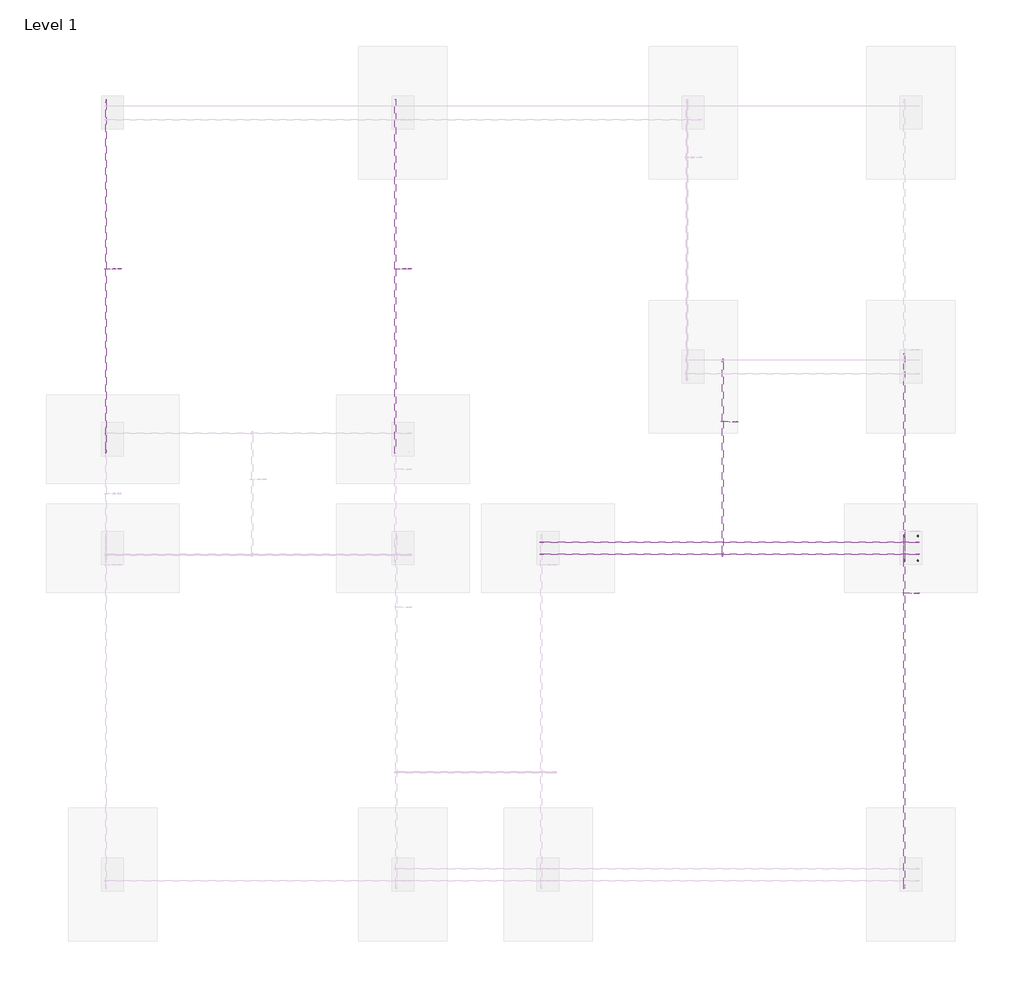
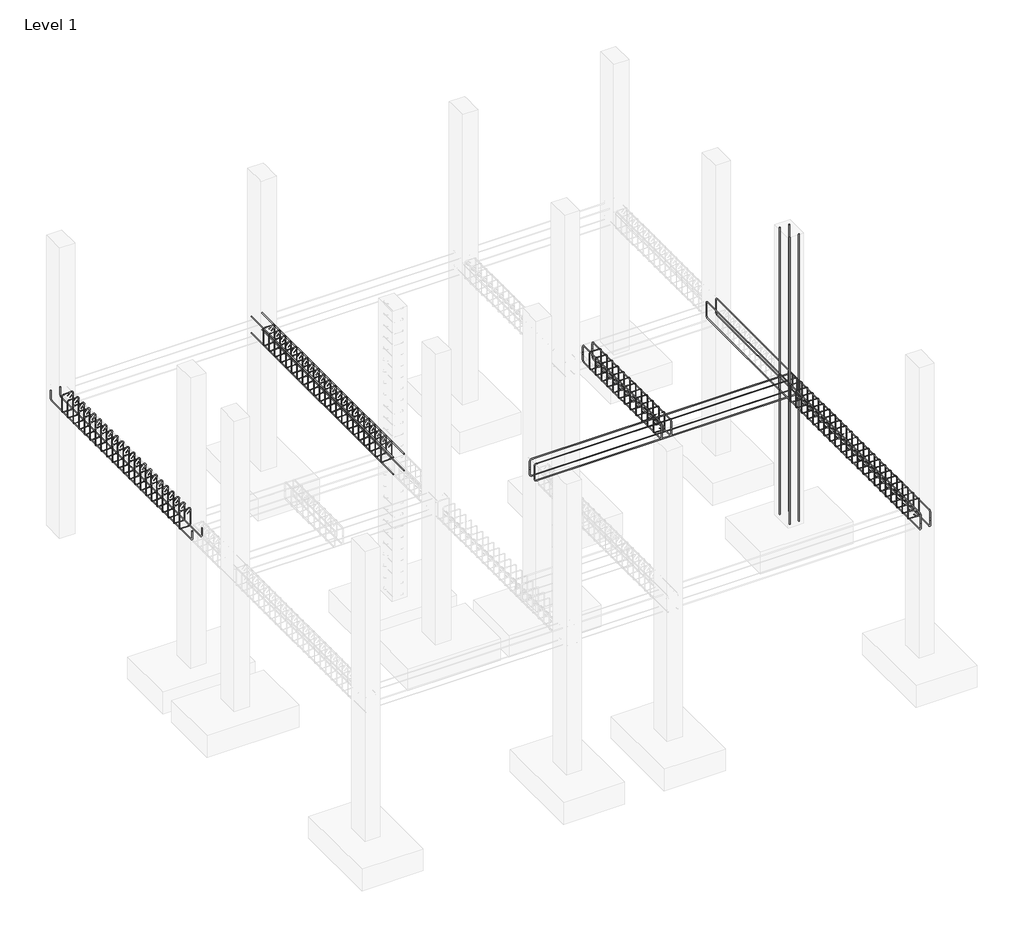
# One storey, part 4 of 5: 17 reinforcing bars.
"""IFC4 building model written with IfcOpenShell, lengths in millimetres."""

from ifc_helpers import new_model, si_unit, point, frame, origin, place, context, project, spatial, polyline, circle_curve, trimmed, segment, composite_curve, source, transform, mapped, element, save
from ifc_brep_helpers import swept_disk

model = new_model("IFC4")

# Units and contexts
model_context = context("Model", 3, world=origin())
ifc_project = project(units=[si_unit("LENGTHUNIT", "METRE", prefix="MILLI")], contexts=[model_context])

# Site, building, storey
site = spatial("IfcSite", under=ifc_project)
building = spatial("IfcBuilding", under=site)
storey = spatial("IfcBuildingStorey", under=building, Name="Level 1", Elevation=0.0)

# Reinforcing bars
placement = place(None, origin())
reinforcing_bar_shape = source(origin(), model_context, "Body", "SolidModel", [
    swept_disk(composite_curve([segment(polyline([(-4212.455746, 5062.3577522, 2793.8967919), (-4212.455746, 5062.3577522, 2946.2967919)]), True, "CONTINUOUS"), segment(trimmed(circle_curve(frame((-4212.455746, 5018.2887522, 2946.2967919), z_axis=(1.0, 0.0, 0.0), x_axis=(0.0, 44.068999999999505, 0.0)), 44.069), [point((-4212.455746, 5062.3577522, 2946.2967919))], [point((-4212.455746, 5018.2887522, 2990.3657919))], True, "CARTESIAN"), True, "CONTINUOUS"), segment(polyline([(-4212.455746, 5018.2887522, 2990.3657919), (-4212.455746, 2237.3647522, 2990.3657919)]), True, "CONTINUOUS"), segment(trimmed(circle_curve(frame((-4212.455746, 2237.3647522, 2946.2967919), z_axis=(1.0, 0.0, 0.0), x_axis=(0.0, 0.0, 44.069000000000415)), 44.069), [point((-4212.455746, 2237.3647522, 2990.3657919))], [point((-4212.455746, 2193.2957522, 2946.2967919))], True, "CARTESIAN"), True, "CONTINUOUS"), segment(polyline([(-4212.455746, 2193.2957522, 2946.2967919), (-4212.455746, 2193.2957522, 2793.8967919)]), True, "CONTINUOUS")], self_intersect=False), 5.969),
])
element("IfcReinforcingBar", 1, at=placement, inside=storey, context=model_context, shape_type="MappedRepresentation", body=[
    mapped(reinforcing_bar_shape, transform((0.0, 0.0, 0.0), x_axis=(1.0, 0.0, 0.0), y_axis=(0.0, 1.0, 0.0), z_axis=(0.0, 0.0, 1.0))),
    mapped(reinforcing_bar_shape, transform((-189.5315837, 0.0, 0.0), x_axis=(1.0, 0.0, 0.0), y_axis=(0.0, 1.0, 0.0), z_axis=(0.0, 0.0, 1.0))),
])
reinforcing_bar_2_shape = source(origin(), model_context, "Body", "SolidModel", [
    swept_disk(composite_curve([segment(polyline([(-4212.455746, 2193.2957522, 2844.9032081), (-4212.455746, 2193.2957522, 2692.5032081)]), True, "CONTINUOUS"), segment(trimmed(circle_curve(frame((-4212.455746, 2237.3647522, 2692.5032081), z_axis=(1.0, 0.0, 0.0), x_axis=(0.0, -44.06899999999996, 0.0)), 44.069), [point((-4212.455746, 2193.2957522, 2692.5032081))], [point((-4212.455746, 2237.3647522, 2648.4342081))], True, "CARTESIAN"), True, "CONTINUOUS"), segment(polyline([(-4212.455746, 2237.3647522, 2648.4342081), (-4212.455746, 5018.2887522, 2648.4342081)]), True, "CONTINUOUS"), segment(trimmed(circle_curve(frame((-4212.455746, 5018.2887522, 2692.5032081), z_axis=(1.0, 0.0, 0.0), x_axis=(0.0, 0.0, -44.06899999999996)), 44.069), [point((-4212.455746, 5018.2887522, 2648.4342081))], [point((-4212.455746, 5062.3577522, 2692.5032081))], True, "CARTESIAN"), True, "CONTINUOUS"), segment(polyline([(-4212.455746, 5062.3577522, 2692.5032081), (-4212.455746, 5062.3577522, 2844.9032081)]), True, "CONTINUOUS")], self_intersect=False), 5.969),
])
element("IfcReinforcingBar", 2, at=placement, inside=storey, context=model_context, shape_type="MappedRepresentation", body=[
    mapped(reinforcing_bar_2_shape, transform((0.0, 0.0, 0.0), x_axis=(1.0, 0.0, 0.0), y_axis=(0.0, 1.0, 0.0), z_axis=(0.0, 0.0, 1.0))),
    mapped(reinforcing_bar_2_shape, transform((-189.5315837, 0.0, 0.0), x_axis=(1.0, 0.0, 0.0), y_axis=(0.0, 1.0, 0.0), z_axis=(0.0, 0.0, 1.0))),
])
reinforcing_bar_3_shape = source(origin(), model_context, "Body", "SolidModel", [
    swept_disk(composite_curve([segment(polyline([(-4212.455746, 2562.3577522, 2793.8967919), (-4212.455746, 2562.3577522, 2946.2967919)]), True, "CONTINUOUS"), segment(trimmed(circle_curve(frame((-4212.455746, 2518.2887522, 2946.2967919), z_axis=(1.0, 0.0, 0.0), x_axis=(0.0, 44.06899999999996, 0.0)), 44.069), [point((-4212.455746, 2562.3577522, 2946.2967919))], [point((-4212.455746, 2518.2887522, 2990.3657919))], True, "CARTESIAN"), True, "CONTINUOUS"), segment(polyline([(-4212.455746, 2518.2887522, 2990.3657919), (-4212.455746, -2262.6352478, 2990.3657919)]), True, "CONTINUOUS"), segment(trimmed(circle_curve(frame((-4212.455746, -2262.6352478, 2946.2967919), z_axis=(1.0, 0.0, 0.0), x_axis=(0.0, 0.0, 44.069000000000415)), 44.069), [point((-4212.455746, -2262.6352478, 2990.3657919))], [point((-4212.455746, -2306.7042478, 2946.2967919))], True, "CARTESIAN"), True, "CONTINUOUS"), segment(polyline([(-4212.455746, -2306.7042478, 2946.2967919), (-4212.455746, -2306.7042478, 2793.8967919)]), True, "CONTINUOUS")], self_intersect=False), 5.969),
])
element("IfcReinforcingBar", 3, at=placement, inside=storey, context=model_context, shape_type="MappedRepresentation", body=[
    mapped(reinforcing_bar_3_shape, transform((0.0, 0.0, 0.0), x_axis=(1.0, 0.0, 0.0), y_axis=(0.0, 1.0, 0.0), z_axis=(0.0, 0.0, 1.0))),
    mapped(reinforcing_bar_3_shape, transform((-189.5315837, 0.0, 0.0), x_axis=(1.0, 0.0, 0.0), y_axis=(0.0, 1.0, 0.0), z_axis=(0.0, 0.0, 1.0))),
])
reinforcing_bar_4_shape = source(origin(), model_context, "Body", "SolidModel", [
    swept_disk(composite_curve([segment(polyline([(-4212.455746, -2306.7042478, 2844.9032081), (-4212.455746, -2306.7042478, 2692.5032081)]), True, "CONTINUOUS"), segment(trimmed(circle_curve(frame((-4212.455746, -2262.6352478, 2692.5032081), z_axis=(1.0, 0.0, 0.0), x_axis=(0.0, -44.06899999999996, 0.0)), 44.069), [point((-4212.455746, -2306.7042478, 2692.5032081))], [point((-4212.455746, -2262.6352478, 2648.4342081))], True, "CARTESIAN"), True, "CONTINUOUS"), segment(polyline([(-4212.455746, -2262.6352478, 2648.4342081), (-4212.455746, 2518.2887522, 2648.4342081)]), True, "CONTINUOUS"), segment(trimmed(circle_curve(frame((-4212.455746, 2518.2887522, 2692.5032081), z_axis=(1.0, 0.0, 0.0), x_axis=(0.0, 0.0, -44.06899999999996)), 44.069), [point((-4212.455746, 2518.2887522, 2648.4342081))], [point((-4212.455746, 2562.3577522, 2692.5032081))], True, "CARTESIAN"), True, "CONTINUOUS"), segment(polyline([(-4212.455746, 2562.3577522, 2692.5032081), (-4212.455746, 2562.3577522, 2844.9032081)]), True, "CONTINUOUS")], self_intersect=False), 5.969),
])
element("IfcReinforcingBar", 4, at=placement, inside=storey, context=model_context, shape_type="MappedRepresentation", body=[
    mapped(reinforcing_bar_4_shape, transform((0.0, 0.0, 0.0), x_axis=(1.0, 0.0, 0.0), y_axis=(0.0, 1.0, 0.0), z_axis=(0.0, 0.0, 1.0))),
    mapped(reinforcing_bar_4_shape, transform((-189.5315837, 0.0, 0.0), x_axis=(1.0, 0.0, 0.0), y_axis=(0.0, 1.0, 0.0), z_axis=(0.0, 0.0, 1.0))),
])
reinforcing_bar_5_shape = source(origin(), model_context, "Body", "SolidModel", [
    swept_disk(composite_curve([segment(polyline([(-4213.892587, 2547.3557031, 38.1), (-4213.892587, 2547.3557031, 6057.9)]), True, "CONTINUOUS")], self_intersect=False), 8.001),
])
element("IfcReinforcingBar", 5, at=placement, inside=storey, context=model_context, shape_type="MappedRepresentation", body=[
    mapped(reinforcing_bar_5_shape, transform((0.0, 0.0, 0.0), x_axis=(1.0, 0.0, 0.0), y_axis=(0.0, 1.0, 0.0), z_axis=(0.0, 0.0, 1.0))),
    mapped(reinforcing_bar_5_shape, transform((-186.6579018, 0.0, 0.0), x_axis=(1.0, 0.0, 0.0), y_axis=(0.0, 1.0, 0.0), z_axis=(0.0, 0.0, 1.0))),
])
reinforcing_bar_6_shape = source(origin(), model_context, "Body", "SolidModel", [
    swept_disk(composite_curve([segment(polyline([(-4213.892587, 2208.2978013, 6057.9), (-4213.892587, 2208.2978013, 38.1)]), True, "CONTINUOUS")], self_intersect=False), 8.001),
])
element("IfcReinforcingBar", 6, at=placement, inside=storey, context=model_context, shape_type="MappedRepresentation", body=[
    mapped(reinforcing_bar_6_shape, transform((0.0, 0.0, 0.0), x_axis=(1.0, 0.0, 0.0), y_axis=(0.0, 1.0, 0.0), z_axis=(0.0, 0.0, 1.0))),
    mapped(reinforcing_bar_6_shape, transform((-186.6579018, 0.0, 0.0), x_axis=(1.0, 0.0, 0.0), y_axis=(0.0, 1.0, 0.0), z_axis=(0.0, 0.0, 1.0))),
])
reinforcing_bar_7_shape = source(origin(), model_context, "Body", "SolidModel", [
    swept_disk(composite_curve([segment(polyline([(-4260.3161447, -1889.6362478, 2737.7833901), (-4205.4511463, -1889.6362478, 2682.9183916)]), True, "CONTINUOUS"), segment(trimmed(circle_curve(frame((-4226.1955379, -1889.6362478, 2662.174), z_axis=(0.0, 1.0, 0.0), x_axis=(20.7443916000002, 0.0, 20.7443916000002)), 29.337), [point((-4205.4511463, -1889.6362478, 2682.9183916))], [point((-4226.1955379, -1889.6362478, 2632.837))], True, "CARTESIAN"), True, "CONTINUOUS"), segment(polyline([(-4226.1955379, -1889.6362478, 2632.837), (-4388.2475379, -1889.6362478, 2632.837)]), True, "CONTINUOUS"), segment(trimmed(circle_curve(frame((-4388.2475379, -1889.6362478, 2662.174), z_axis=(0.0, 1.0, 0.0), x_axis=(0.0, 0.0, -29.33699999999999)), 29.337), [point((-4388.2475379, -1889.6362478, 2632.837))], [point((-4417.5845379, -1889.6362478, 2662.174))], True, "CARTESIAN"), True, "CONTINUOUS"), segment(polyline([(-4417.5845379, -1889.6362478, 2662.174), (-4417.5845379, -1889.6362478, 2976.626)]), True, "CONTINUOUS"), segment(trimmed(circle_curve(frame((-4388.2661869, -1890.6821269, 2976.626), z_axis=(0.03565051078635361, 0.9993643184948481, 0.0), x_axis=(-29.318350999999893, 1.0458790999998655, 0.0)), 29.337), [point((-4417.5845379, -1889.6362478, 2976.626))], [point((-4388.2661869, -1890.6821269, 3005.963))], True, "CARTESIAN"), True, "CONTINUOUS"), segment(polyline([(-4388.2661869, -1890.6821269, 3005.963), (-4226.1768889, -1896.4643688, 3005.963)]), True, "CONTINUOUS"), segment(trimmed(circle_curve(frame((-4226.1768889, -1896.4643688, 2976.626), z_axis=(0.03565051078635361, 0.9993643184948481, 0.0), x_axis=(0.0, 0.0, 29.33699999999999)), 29.337), [point((-4226.1768889, -1896.4643688, 3005.963))], [point((-4196.8585379, -1897.5102478, 2976.626))], True, "CARTESIAN"), True, "CONTINUOUS"), segment(polyline([(-4196.8585379, -1897.5102478, 2976.626), (-4196.8585379, -1897.5102478, 2662.174)]), True, "CONTINUOUS"), segment(trimmed(circle_curve(frame((-4226.1955379, -1897.5102478, 2662.174), z_axis=(0.0, 1.0, 0.0), x_axis=(29.337000000000444, 0.0, 0.0)), 29.337), [point((-4196.8585379, -1897.5102478, 2662.174))], [point((-4246.9399295, -1897.5102478, 2641.4296084))], True, "CARTESIAN"), True, "CONTINUOUS"), segment(polyline([(-4246.9399295, -1897.5102478, 2641.4296084), (-4301.804928, -1897.5102478, 2696.2946068)]), True, "CONTINUOUS")], self_intersect=False), 3.937),
])
element("IfcReinforcingBar", 7, at=placement, inside=storey, context=model_context, shape_type="MappedRepresentation", body=[
    mapped(reinforcing_bar_7_shape, transform((0.0, 0.0, 0.0), x_axis=(1.0, 0.0, 0.0), y_axis=(0.0, 1.0, 0.0), z_axis=(0.0, 0.0, 1.0))),
    mapped(reinforcing_bar_7_shape, transform((0.0, 192.1393333, 0.0), x_axis=(1.0, 0.0, 0.0), y_axis=(0.0, 1.0, 0.0), z_axis=(0.0, 0.0, 1.0))),
    mapped(reinforcing_bar_7_shape, transform((0.0, 384.2786667, 0.0), x_axis=(1.0, 0.0, 0.0), y_axis=(0.0, 1.0, 0.0), z_axis=(0.0, 0.0, 1.0))),
    mapped(reinforcing_bar_7_shape, transform((0.0, 576.418, 0.0), x_axis=(1.0, 0.0, 0.0), y_axis=(0.0, 1.0, 0.0), z_axis=(0.0, 0.0, 1.0))),
    mapped(reinforcing_bar_7_shape, transform((0.0, 768.5573333, 0.0), x_axis=(1.0, 0.0, 0.0), y_axis=(0.0, 1.0, 0.0), z_axis=(0.0, 0.0, 1.0))),
    mapped(reinforcing_bar_7_shape, transform((0.0, 960.6966667, 0.0), x_axis=(1.0, 0.0, 0.0), y_axis=(0.0, 1.0, 0.0), z_axis=(0.0, 0.0, 1.0))),
    mapped(reinforcing_bar_7_shape, transform((0.0, 1152.836, 0.0), x_axis=(1.0, 0.0, 0.0), y_axis=(0.0, 1.0, 0.0), z_axis=(0.0, 0.0, 1.0))),
    mapped(reinforcing_bar_7_shape, transform((0.0, 1344.9753333, 0.0), x_axis=(1.0, 0.0, 0.0), y_axis=(0.0, 1.0, 0.0), z_axis=(0.0, 0.0, 1.0))),
    mapped(reinforcing_bar_7_shape, transform((0.0, 1537.1146667, 0.0), x_axis=(1.0, 0.0, 0.0), y_axis=(0.0, 1.0, 0.0), z_axis=(0.0, 0.0, 1.0))),
    mapped(reinforcing_bar_7_shape, transform((0.0, 1729.254, 0.0), x_axis=(1.0, 0.0, 0.0), y_axis=(0.0, 1.0, 0.0), z_axis=(0.0, 0.0, 1.0))),
    mapped(reinforcing_bar_7_shape, transform((0.0, 1921.3933333, 0.0), x_axis=(1.0, 0.0, 0.0), y_axis=(0.0, 1.0, 0.0), z_axis=(0.0, 0.0, 1.0))),
    mapped(reinforcing_bar_7_shape, transform((0.0, 2113.5326667, 0.0), x_axis=(1.0, 0.0, 0.0), y_axis=(0.0, 1.0, 0.0), z_axis=(0.0, 0.0, 1.0))),
    mapped(reinforcing_bar_7_shape, transform((0.0, 2305.672, 0.0), x_axis=(1.0, 0.0, 0.0), y_axis=(0.0, 1.0, 0.0), z_axis=(0.0, 0.0, 1.0))),
    mapped(reinforcing_bar_7_shape, transform((0.0, 2497.8113333, 0.0), x_axis=(1.0, 0.0, 0.0), y_axis=(0.0, 1.0, 0.0), z_axis=(0.0, 0.0, 1.0))),
    mapped(reinforcing_bar_7_shape, transform((0.0, 2689.9506667, 0.0), x_axis=(1.0, 0.0, 0.0), y_axis=(0.0, 1.0, 0.0), z_axis=(0.0, 0.0, 1.0))),
    mapped(reinforcing_bar_7_shape, transform((0.0, 2882.09, 0.0), x_axis=(1.0, 0.0, 0.0), y_axis=(0.0, 1.0, 0.0), z_axis=(0.0, 0.0, 1.0))),
    mapped(reinforcing_bar_7_shape, transform((0.0, 3074.2293333, 0.0), x_axis=(1.0, 0.0, 0.0), y_axis=(0.0, 1.0, 0.0), z_axis=(0.0, 0.0, 1.0))),
    mapped(reinforcing_bar_7_shape, transform((0.0, 3266.3686667, 0.0), x_axis=(1.0, 0.0, 0.0), y_axis=(0.0, 1.0, 0.0), z_axis=(0.0, 0.0, 1.0))),
    mapped(reinforcing_bar_7_shape, transform((0.0, 3458.508, 0.0), x_axis=(1.0, 0.0, 0.0), y_axis=(0.0, 1.0, 0.0), z_axis=(0.0, 0.0, 1.0))),
    mapped(reinforcing_bar_7_shape, transform((0.0, 3650.6473333, 0.0), x_axis=(1.0, 0.0, 0.0), y_axis=(0.0, 1.0, 0.0), z_axis=(0.0, 0.0, 1.0))),
    mapped(reinforcing_bar_7_shape, transform((0.0, 3842.7866667, 0.0), x_axis=(1.0, 0.0, 0.0), y_axis=(0.0, 1.0, 0.0), z_axis=(0.0, 0.0, 1.0))),
    mapped(reinforcing_bar_7_shape, transform((0.0, 4034.926, 0.0), x_axis=(1.0, 0.0, 0.0), y_axis=(0.0, 1.0, 0.0), z_axis=(0.0, 0.0, 1.0))),
])
reinforcing_bar_8_shape = source(origin(), model_context, "Body", "SolidModel", [
    swept_disk(composite_curve([segment(polyline([(-15212.455746, 3693.2957522, 2844.9032081), (-15212.455746, 3693.2957522, 2692.5032081)]), True, "CONTINUOUS"), segment(trimmed(circle_curve(frame((-15212.455746, 3737.3647522, 2692.5032081), z_axis=(1.0, 0.0, 0.0), x_axis=(0.0, -44.06899999999996, 0.0)), 44.069), [point((-15212.455746, 3693.2957522, 2692.5032081))], [point((-15212.455746, 3737.3647522, 2648.4342081))], True, "CARTESIAN"), True, "CONTINUOUS"), segment(polyline([(-15212.455746, 3737.3647522, 2648.4342081), (-15212.455746, 8518.2887522, 2648.4342081)]), True, "CONTINUOUS"), segment(trimmed(circle_curve(frame((-15212.455746, 8518.2887522, 2692.5032081), z_axis=(1.0, 0.0, 0.0), x_axis=(0.0, 0.0, -44.06899999999996)), 44.069), [point((-15212.455746, 8518.2887522, 2648.4342081))], [point((-15212.455746, 8562.3577522, 2692.5032081))], True, "CARTESIAN"), True, "CONTINUOUS"), segment(polyline([(-15212.455746, 8562.3577522, 2692.5032081), (-15212.455746, 8562.3577522, 2844.9032081)]), True, "CONTINUOUS")], self_intersect=False), 5.969),
])
element("IfcReinforcingBar", 8, at=placement, inside=storey, context=model_context, shape_type="MappedRepresentation", body=[
    mapped(reinforcing_bar_8_shape, transform((0.0, 0.0, 0.0), x_axis=(1.0, 0.0, 0.0), y_axis=(0.0, 1.0, 0.0), z_axis=(0.0, 0.0, 1.0))),
    mapped(reinforcing_bar_8_shape, transform((-189.5315837, 0.0, 0.0), x_axis=(1.0, 0.0, 0.0), y_axis=(0.0, 1.0, 0.0), z_axis=(0.0, 0.0, 1.0))),
])
reinforcing_bar_9_shape = source(origin(), model_context, "Body", "SolidModel", [
    swept_disk(composite_curve([segment(polyline([(-15260.3161447, 8145.2897522, 2901.0166099), (-15205.4511463, 8145.2897522, 2955.8816084)]), True, "CONTINUOUS"), segment(trimmed(circle_curve(frame((-15226.1955379, 8145.2897522, 2976.626), z_axis=(0.0, -1.0, 0.0), x_axis=(20.74439159999929, 0.0, -20.7443916000002)), 29.337), [point((-15205.4511463, 8145.2897522, 2955.8816084))], [point((-15226.1955379, 8145.2897522, 3005.963))], True, "CARTESIAN"), True, "CONTINUOUS"), segment(polyline([(-15226.1955379, 8145.2897522, 3005.963), (-15388.2475379, 8145.2897522, 3005.963)]), True, "CONTINUOUS"), segment(trimmed(circle_curve(frame((-15388.2475379, 8145.2897522, 2976.626), z_axis=(0.0, -1.0, 0.0), x_axis=(0.0, 0.0, 29.33699999999999)), 29.337), [point((-15388.2475379, 8145.2897522, 3005.963))], [point((-15417.5845379, 8145.2897522, 2976.626))], True, "CARTESIAN"), True, "CONTINUOUS"), segment(polyline([(-15417.5845379, 8145.2897522, 2976.626), (-15417.5845379, 8145.2897522, 2662.174)]), True, "CONTINUOUS"), segment(trimmed(circle_curve(frame((-15388.2661869, 8146.3356312, 2662.174), z_axis=(0.03565051078635043, -0.9993643184948482, 0.0), x_axis=(-29.318350999999893, -1.0458789999993314, 0.0)), 29.337), [point((-15417.5845379, 8145.2897522, 2662.174))], [point((-15388.2661869, 8146.3356312, 2632.837))], True, "CARTESIAN"), True, "CONTINUOUS"), segment(polyline([(-15388.2661869, 8146.3356312, 2632.837), (-15226.1768889, 8152.1178731, 2632.837)]), True, "CONTINUOUS"), segment(trimmed(circle_curve(frame((-15226.1768889, 8152.1178731, 2662.174), z_axis=(0.03565051078635043, -0.9993643184948482, 0.0), x_axis=(0.0, 0.0, -29.33699999999999)), 29.337), [point((-15226.1768889, 8152.1178731, 2632.837))], [point((-15196.8585379, 8153.1637522, 2662.174))], True, "CARTESIAN"), True, "CONTINUOUS"), segment(polyline([(-15196.8585379, 8153.1637522, 2662.174), (-15196.8585379, 8153.1637522, 2976.626)]), True, "CONTINUOUS"), segment(trimmed(circle_curve(frame((-15226.1955379, 8153.1637522, 2976.626), z_axis=(0.0, -1.0, 0.0), x_axis=(29.336999999999534, 0.0, 0.0)), 29.337), [point((-15196.8585379, 8153.1637522, 2976.626))], [point((-15246.9399295, 8153.1637522, 2997.3703916))], True, "CARTESIAN"), True, "CONTINUOUS"), segment(polyline([(-15246.9399295, 8153.1637522, 2997.3703916), (-15301.804928, 8153.1637522, 2942.5053932)]), True, "CONTINUOUS")], self_intersect=False), 3.937),
])
element("IfcReinforcingBar", 9, at=placement, inside=storey, context=model_context, shape_type="MappedRepresentation", body=[
    mapped(reinforcing_bar_9_shape, transform((0.0, 0.0, 0.0), x_axis=(1.0, 0.0, 0.0), y_axis=(0.0, 1.0, 0.0), z_axis=(0.0, 0.0, 1.0))),
    mapped(reinforcing_bar_9_shape, transform((0.0, -192.1393333, 0.0), x_axis=(1.0, 0.0, 0.0), y_axis=(0.0, 1.0, 0.0), z_axis=(0.0, 0.0, 1.0))),
    mapped(reinforcing_bar_9_shape, transform((0.0, -384.2786667, 0.0), x_axis=(1.0, 0.0, 0.0), y_axis=(0.0, 1.0, 0.0), z_axis=(0.0, 0.0, 1.0))),
    mapped(reinforcing_bar_9_shape, transform((0.0, -576.418, 0.0), x_axis=(1.0, 0.0, 0.0), y_axis=(0.0, 1.0, 0.0), z_axis=(0.0, 0.0, 1.0))),
    mapped(reinforcing_bar_9_shape, transform((0.0, -768.5573333, 0.0), x_axis=(1.0, 0.0, 0.0), y_axis=(0.0, 1.0, 0.0), z_axis=(0.0, 0.0, 1.0))),
    mapped(reinforcing_bar_9_shape, transform((0.0, -960.6966667, 0.0), x_axis=(1.0, 0.0, 0.0), y_axis=(0.0, 1.0, 0.0), z_axis=(0.0, 0.0, 1.0))),
    mapped(reinforcing_bar_9_shape, transform((0.0, -1152.836, 0.0), x_axis=(1.0, 0.0, 0.0), y_axis=(0.0, 1.0, 0.0), z_axis=(0.0, 0.0, 1.0))),
    mapped(reinforcing_bar_9_shape, transform((0.0, -1344.9753333, 0.0), x_axis=(1.0, 0.0, 0.0), y_axis=(0.0, 1.0, 0.0), z_axis=(0.0, 0.0, 1.0))),
    mapped(reinforcing_bar_9_shape, transform((0.0, -1537.1146667, 0.0), x_axis=(1.0, 0.0, 0.0), y_axis=(0.0, 1.0, 0.0), z_axis=(0.0, 0.0, 1.0))),
    mapped(reinforcing_bar_9_shape, transform((0.0, -1729.254, 0.0), x_axis=(1.0, 0.0, 0.0), y_axis=(0.0, 1.0, 0.0), z_axis=(0.0, 0.0, 1.0))),
    mapped(reinforcing_bar_9_shape, transform((0.0, -1921.3933333, 0.0), x_axis=(1.0, 0.0, 0.0), y_axis=(0.0, 1.0, 0.0), z_axis=(0.0, 0.0, 1.0))),
    mapped(reinforcing_bar_9_shape, transform((0.0, -2113.5326667, 0.0), x_axis=(1.0, 0.0, 0.0), y_axis=(0.0, 1.0, 0.0), z_axis=(0.0, 0.0, 1.0))),
    mapped(reinforcing_bar_9_shape, transform((0.0, -2305.672, 0.0), x_axis=(1.0, 0.0, 0.0), y_axis=(0.0, 1.0, 0.0), z_axis=(0.0, 0.0, 1.0))),
    mapped(reinforcing_bar_9_shape, transform((0.0, -2497.8113333, 0.0), x_axis=(1.0, 0.0, 0.0), y_axis=(0.0, 1.0, 0.0), z_axis=(0.0, 0.0, 1.0))),
    mapped(reinforcing_bar_9_shape, transform((0.0, -2689.9506667, 0.0), x_axis=(1.0, 0.0, 0.0), y_axis=(0.0, 1.0, 0.0), z_axis=(0.0, 0.0, 1.0))),
    mapped(reinforcing_bar_9_shape, transform((0.0, -2882.09, 0.0), x_axis=(1.0, 0.0, 0.0), y_axis=(0.0, 1.0, 0.0), z_axis=(0.0, 0.0, 1.0))),
    mapped(reinforcing_bar_9_shape, transform((0.0, -3074.2293333, 0.0), x_axis=(1.0, 0.0, 0.0), y_axis=(0.0, 1.0, 0.0), z_axis=(0.0, 0.0, 1.0))),
    mapped(reinforcing_bar_9_shape, transform((0.0, -3266.3686667, 0.0), x_axis=(1.0, 0.0, 0.0), y_axis=(0.0, 1.0, 0.0), z_axis=(0.0, 0.0, 1.0))),
    mapped(reinforcing_bar_9_shape, transform((0.0, -3458.508, 0.0), x_axis=(1.0, 0.0, 0.0), y_axis=(0.0, 1.0, 0.0), z_axis=(0.0, 0.0, 1.0))),
    mapped(reinforcing_bar_9_shape, transform((0.0, -3650.6473333, 0.0), x_axis=(1.0, 0.0, 0.0), y_axis=(0.0, 1.0, 0.0), z_axis=(0.0, 0.0, 1.0))),
    mapped(reinforcing_bar_9_shape, transform((0.0, -3842.7866667, 0.0), x_axis=(1.0, 0.0, 0.0), y_axis=(0.0, 1.0, 0.0), z_axis=(0.0, 0.0, 1.0))),
    mapped(reinforcing_bar_9_shape, transform((0.0, -4034.926, 0.0), x_axis=(1.0, 0.0, 0.0), y_axis=(0.0, 1.0, 0.0), z_axis=(0.0, 0.0, 1.0))),
])
reinforcing_bar_10_shape = source(origin(), model_context, "Body", "SolidModel", [
    swept_disk(composite_curve([segment(polyline([(-11198.8905379, 8568.3267522, 2996.057), (-11198.8905379, 3687.3267522, 2996.057)]), True, "CONTINUOUS")], self_intersect=False), 5.969),
])
element("IfcReinforcingBar", 10, at=placement, inside=storey, context=model_context, shape_type="MappedRepresentation", body=[
    mapped(reinforcing_bar_10_shape, transform((0.0, 0.0, 0.0), x_axis=(1.0, 0.0, 0.0), y_axis=(0.0, 1.0, 0.0), z_axis=(0.0, 0.0, 1.0))),
    mapped(reinforcing_bar_10_shape, transform((-216.662, 0.0, 0.0), x_axis=(1.0, 0.0, 0.0), y_axis=(0.0, 1.0, 0.0), z_axis=(0.0, 0.0, 1.0))),
])
reinforcing_bar_11_shape = source(origin(), model_context, "Body", "SolidModel", [
    swept_disk(composite_curve([segment(polyline([(-11198.8905379, 3687.3267522, 2642.743), (-11198.8905379, 8568.3267522, 2642.743)]), True, "CONTINUOUS")], self_intersect=False), 5.969),
])
element("IfcReinforcingBar", 11, at=placement, inside=storey, context=model_context, shape_type="MappedRepresentation", body=[
    mapped(reinforcing_bar_11_shape, transform((0.0, 0.0, 0.0), x_axis=(1.0, 0.0, 0.0), y_axis=(0.0, 1.0, 0.0), z_axis=(0.0, 0.0, 1.0))),
    mapped(reinforcing_bar_11_shape, transform((-216.662, 0.0, 0.0), x_axis=(1.0, 0.0, 0.0), y_axis=(0.0, 1.0, 0.0), z_axis=(0.0, 0.0, 1.0))),
])
reinforcing_bar_12_shape = source(origin(), model_context, "Body", "SolidModel", [
    swept_disk(composite_curve([segment(polyline([(-11260.3161447, 8145.2897522, 2901.0166099), (-11205.4511463, 8145.2897522, 2955.8816084)]), True, "CONTINUOUS"), segment(trimmed(circle_curve(frame((-11226.1955379, 8145.2897522, 2976.626), z_axis=(0.0, -1.0, 0.0), x_axis=(20.74439159999929, 0.0, -20.7443916000002)), 29.337), [point((-11205.4511463, 8145.2897522, 2955.8816084))], [point((-11226.1955379, 8145.2897522, 3005.963))], True, "CARTESIAN"), True, "CONTINUOUS"), segment(polyline([(-11226.1955379, 8145.2897522, 3005.963), (-11388.2475379, 8145.2897522, 3005.963)]), True, "CONTINUOUS"), segment(trimmed(circle_curve(frame((-11388.2475379, 8145.2897522, 2976.626), z_axis=(0.0, -1.0, 0.0), x_axis=(0.0, 0.0, 29.33699999999999)), 29.337), [point((-11388.2475379, 8145.2897522, 3005.963))], [point((-11417.5845379, 8145.2897522, 2976.626))], True, "CARTESIAN"), True, "CONTINUOUS"), segment(polyline([(-11417.5845379, 8145.2897522, 2976.626), (-11417.5845379, 8145.2897522, 2662.174)]), True, "CONTINUOUS"), segment(trimmed(circle_curve(frame((-11388.2661869, 8146.3356312, 2662.174), z_axis=(0.035650510786351154, -0.9993643184948482, 0.0), x_axis=(-29.318350999999893, -1.0458789999993314, 0.0)), 29.337), [point((-11417.5845379, 8145.2897522, 2662.174))], [point((-11388.2661869, 8146.3356312, 2632.837))], True, "CARTESIAN"), True, "CONTINUOUS"), segment(polyline([(-11388.2661869, 8146.3356312, 2632.837), (-11226.1768889, 8152.1178731, 2632.837)]), True, "CONTINUOUS"), segment(trimmed(circle_curve(frame((-11226.1768889, 8152.1178731, 2662.174), z_axis=(0.035650510786351154, -0.9993643184948482, 0.0), x_axis=(0.0, 0.0, -29.33699999999999)), 29.337), [point((-11226.1768889, 8152.1178731, 2632.837))], [point((-11196.8585379, 8153.1637522, 2662.174))], True, "CARTESIAN"), True, "CONTINUOUS"), segment(polyline([(-11196.8585379, 8153.1637522, 2662.174), (-11196.8585379, 8153.1637522, 2976.626)]), True, "CONTINUOUS"), segment(trimmed(circle_curve(frame((-11226.1955379, 8153.1637522, 2976.626), z_axis=(0.0, -1.0, 0.0), x_axis=(29.336999999999534, 0.0, 0.0)), 29.337), [point((-11196.8585379, 8153.1637522, 2976.626))], [point((-11246.9399295, 8153.1637522, 2997.3703916))], True, "CARTESIAN"), True, "CONTINUOUS"), segment(polyline([(-11246.9399295, 8153.1637522, 2997.3703916), (-11301.804928, 8153.1637522, 2942.5053932)]), True, "CONTINUOUS")], self_intersect=False), 3.937),
])
element("IfcReinforcingBar", 12, at=placement, inside=storey, context=model_context, shape_type="MappedRepresentation", body=[
    mapped(reinforcing_bar_12_shape, transform((0.0, 0.0, 0.0), x_axis=(1.0, 0.0, 0.0), y_axis=(0.0, 1.0, 0.0), z_axis=(0.0, 0.0, 1.0))),
    mapped(reinforcing_bar_12_shape, transform((0.0, -192.1393333, 0.0), x_axis=(1.0, 0.0, 0.0), y_axis=(0.0, 1.0, 0.0), z_axis=(0.0, 0.0, 1.0))),
    mapped(reinforcing_bar_12_shape, transform((0.0, -384.2786667, 0.0), x_axis=(1.0, 0.0, 0.0), y_axis=(0.0, 1.0, 0.0), z_axis=(0.0, 0.0, 1.0))),
    mapped(reinforcing_bar_12_shape, transform((0.0, -576.418, 0.0), x_axis=(1.0, 0.0, 0.0), y_axis=(0.0, 1.0, 0.0), z_axis=(0.0, 0.0, 1.0))),
    mapped(reinforcing_bar_12_shape, transform((0.0, -768.5573333, 0.0), x_axis=(1.0, 0.0, 0.0), y_axis=(0.0, 1.0, 0.0), z_axis=(0.0, 0.0, 1.0))),
    mapped(reinforcing_bar_12_shape, transform((0.0, -960.6966667, 0.0), x_axis=(1.0, 0.0, 0.0), y_axis=(0.0, 1.0, 0.0), z_axis=(0.0, 0.0, 1.0))),
    mapped(reinforcing_bar_12_shape, transform((0.0, -1152.836, 0.0), x_axis=(1.0, 0.0, 0.0), y_axis=(0.0, 1.0, 0.0), z_axis=(0.0, 0.0, 1.0))),
    mapped(reinforcing_bar_12_shape, transform((0.0, -1344.9753333, 0.0), x_axis=(1.0, 0.0, 0.0), y_axis=(0.0, 1.0, 0.0), z_axis=(0.0, 0.0, 1.0))),
    mapped(reinforcing_bar_12_shape, transform((0.0, -1537.1146667, 0.0), x_axis=(1.0, 0.0, 0.0), y_axis=(0.0, 1.0, 0.0), z_axis=(0.0, 0.0, 1.0))),
    mapped(reinforcing_bar_12_shape, transform((0.0, -1729.254, 0.0), x_axis=(1.0, 0.0, 0.0), y_axis=(0.0, 1.0, 0.0), z_axis=(0.0, 0.0, 1.0))),
    mapped(reinforcing_bar_12_shape, transform((0.0, -1921.3933333, 0.0), x_axis=(1.0, 0.0, 0.0), y_axis=(0.0, 1.0, 0.0), z_axis=(0.0, 0.0, 1.0))),
    mapped(reinforcing_bar_12_shape, transform((0.0, -2113.5326667, 0.0), x_axis=(1.0, 0.0, 0.0), y_axis=(0.0, 1.0, 0.0), z_axis=(0.0, 0.0, 1.0))),
    mapped(reinforcing_bar_12_shape, transform((0.0, -2305.672, 0.0), x_axis=(1.0, 0.0, 0.0), y_axis=(0.0, 1.0, 0.0), z_axis=(0.0, 0.0, 1.0))),
    mapped(reinforcing_bar_12_shape, transform((0.0, -2497.8113333, 0.0), x_axis=(1.0, 0.0, 0.0), y_axis=(0.0, 1.0, 0.0), z_axis=(0.0, 0.0, 1.0))),
    mapped(reinforcing_bar_12_shape, transform((0.0, -2689.9506667, 0.0), x_axis=(1.0, 0.0, 0.0), y_axis=(0.0, 1.0, 0.0), z_axis=(0.0, 0.0, 1.0))),
    mapped(reinforcing_bar_12_shape, transform((0.0, -2882.09, 0.0), x_axis=(1.0, 0.0, 0.0), y_axis=(0.0, 1.0, 0.0), z_axis=(0.0, 0.0, 1.0))),
    mapped(reinforcing_bar_12_shape, transform((0.0, -3074.2293333, 0.0), x_axis=(1.0, 0.0, 0.0), y_axis=(0.0, 1.0, 0.0), z_axis=(0.0, 0.0, 1.0))),
    mapped(reinforcing_bar_12_shape, transform((0.0, -3266.3686667, 0.0), x_axis=(1.0, 0.0, 0.0), y_axis=(0.0, 1.0, 0.0), z_axis=(0.0, 0.0, 1.0))),
    mapped(reinforcing_bar_12_shape, transform((0.0, -3458.508, 0.0), x_axis=(1.0, 0.0, 0.0), y_axis=(0.0, 1.0, 0.0), z_axis=(0.0, 0.0, 1.0))),
    mapped(reinforcing_bar_12_shape, transform((0.0, -3650.6473333, 0.0), x_axis=(1.0, 0.0, 0.0), y_axis=(0.0, 1.0, 0.0), z_axis=(0.0, 0.0, 1.0))),
    mapped(reinforcing_bar_12_shape, transform((0.0, -3842.7866667, 0.0), x_axis=(1.0, 0.0, 0.0), y_axis=(0.0, 1.0, 0.0), z_axis=(0.0, 0.0, 1.0))),
    mapped(reinforcing_bar_12_shape, transform((0.0, -4034.926, 0.0), x_axis=(1.0, 0.0, 0.0), y_axis=(0.0, 1.0, 0.0), z_axis=(0.0, 0.0, 1.0))),
])
reinforcing_bar_13_shape = source(origin(), model_context, "Body", "SolidModel", [
    swept_disk(composite_curve([segment(polyline([(-4198.8905379, 2458.8527522, 2799.588), (-4198.8905379, 2458.8527522, 2951.988)]), True, "CONTINUOUS"), segment(trimmed(circle_curve(frame((-4242.9595379, 2458.8527522, 2951.988), z_axis=(0.0, -1.0, 0.0), x_axis=(44.069000000000415, 0.0, 0.0)), 44.069), [point((-4198.8905379, 2458.8527522, 2951.988))], [point((-4242.9595379, 2458.8527522, 2996.057))], True, "CARTESIAN"), True, "CONTINUOUS"), segment(polyline([(-4242.9595379, 2458.8527522, 2996.057), (-9371.4835379, 2458.8527522, 2996.057)]), True, "CONTINUOUS"), segment(trimmed(circle_curve(frame((-9371.4835379, 2458.8527522, 2951.988), z_axis=(0.0, -1.0, 0.0), x_axis=(0.0, 0.0, 44.06899999999996)), 44.069), [point((-9371.4835379, 2458.8527522, 2996.057))], [point((-9415.5525379, 2458.8527522, 2951.988))], True, "CARTESIAN"), True, "CONTINUOUS"), segment(polyline([(-9415.5525379, 2458.8527522, 2951.988), (-9415.5525379, 2458.8527522, 2799.588)]), True, "CONTINUOUS")], self_intersect=False), 5.969),
])
element("IfcReinforcingBar", 13, at=placement, inside=storey, context=model_context, shape_type="MappedRepresentation", body=[
    mapped(reinforcing_bar_13_shape, transform((0.0, 0.0, 0.0), x_axis=(1.0, 0.0, 0.0), y_axis=(0.0, 1.0, 0.0), z_axis=(0.0, 0.0, 1.0))),
    mapped(reinforcing_bar_13_shape, transform((0.0, -162.052, 0.0), x_axis=(1.0, 0.0, 0.0), y_axis=(0.0, 1.0, 0.0), z_axis=(0.0, 0.0, 1.0))),
])
reinforcing_bar_14_shape = source(origin(), model_context, "Body", "SolidModel", [
    swept_disk(composite_curve([segment(polyline([(-9415.5525379, 2296.8007522, 2839.212), (-9415.5525379, 2296.8007522, 2686.812)]), True, "CONTINUOUS"), segment(trimmed(circle_curve(frame((-9371.4835379, 2296.8007522, 2686.812), z_axis=(0.0, -1.0, 0.0), x_axis=(-44.068999999999505, 0.0, 0.0)), 44.069), [point((-9415.5525379, 2296.8007522, 2686.812))], [point((-9371.4835379, 2296.8007522, 2642.743))], True, "CARTESIAN"), True, "CONTINUOUS"), segment(polyline([(-9371.4835379, 2296.8007522, 2642.743), (-4242.9595379, 2296.8007522, 2642.743)]), True, "CONTINUOUS"), segment(trimmed(circle_curve(frame((-4242.9595379, 2296.8007522, 2686.812), z_axis=(0.0, -1.0, 0.0), x_axis=(0.0, 0.0, -44.06899999999996)), 44.069), [point((-4242.9595379, 2296.8007522, 2642.743))], [point((-4198.8905379, 2296.8007522, 2686.812))], True, "CARTESIAN"), True, "CONTINUOUS"), segment(polyline([(-4198.8905379, 2296.8007522, 2686.812), (-4198.8905379, 2296.8007522, 2839.212)]), True, "CONTINUOUS")], self_intersect=False), 5.969),
])
element("IfcReinforcingBar", 14, at=placement, inside=storey, context=model_context, shape_type="MappedRepresentation", body=[
    mapped(reinforcing_bar_14_shape, transform((0.0, 0.0, 0.0), x_axis=(1.0, 0.0, 0.0), y_axis=(0.0, 1.0, 0.0), z_axis=(0.0, 0.0, 1.0))),
    mapped(reinforcing_bar_14_shape, transform((0.0, 162.052, 0.0), x_axis=(1.0, 0.0, 0.0), y_axis=(0.0, 1.0, 0.0), z_axis=(0.0, 0.0, 1.0))),
])
reinforcing_bar_15_shape = source(origin(), model_context, "Body", "SolidModel", [
    swept_disk(composite_curve([segment(polyline([(-6712.455746, 4986.1577522, 2793.8967919), (-6712.455746, 4986.1577522, 2946.2967919)]), True, "CONTINUOUS"), segment(trimmed(circle_curve(frame((-6712.455746, 4942.0887522, 2946.2967919), z_axis=(1.0, 0.0, 0.0), x_axis=(0.0, 44.068999999999505, 0.0)), 44.069), [point((-6712.455746, 4986.1577522, 2946.2967919))], [point((-6712.455746, 4942.0887522, 2990.3657919))], True, "CARTESIAN"), True, "CONTINUOUS"), segment(polyline([(-6712.455746, 4942.0887522, 2990.3657919), (-6712.455746, 2313.5647522, 2990.3657919)]), True, "CONTINUOUS"), segment(trimmed(circle_curve(frame((-6712.455746, 2313.5647522, 2946.2967919), z_axis=(1.0, 0.0, 0.0), x_axis=(0.0, 0.0, 44.069000000000415)), 44.069), [point((-6712.455746, 2313.5647522, 2990.3657919))], [point((-6712.455746, 2269.4957522, 2946.2967919))], True, "CARTESIAN"), True, "CONTINUOUS"), segment(polyline([(-6712.455746, 2269.4957522, 2946.2967919), (-6712.455746, 2269.4957522, 2793.8967919)]), True, "CONTINUOUS")], self_intersect=False), 5.969),
])
element("IfcReinforcingBar", 15, at=placement, inside=storey, context=model_context, shape_type="MappedRepresentation", body=[
    mapped(reinforcing_bar_15_shape, transform((0.0, 0.0, 0.0), x_axis=(1.0, 0.0, 0.0), y_axis=(0.0, 1.0, 0.0), z_axis=(0.0, 0.0, 1.0))),
    mapped(reinforcing_bar_15_shape, transform((-189.5315837, 0.0, 0.0), x_axis=(1.0, 0.0, 0.0), y_axis=(0.0, 1.0, 0.0), z_axis=(0.0, 0.0, 1.0))),
])
reinforcing_bar_16_shape = source(origin(), model_context, "Body", "SolidModel", [
    swept_disk(composite_curve([segment(polyline([(-6712.455746, 2269.4957522, 2844.9032081), (-6712.455746, 2269.4957522, 2692.5032081)]), True, "CONTINUOUS"), segment(trimmed(circle_curve(frame((-6712.455746, 2313.5647522, 2692.5032081), z_axis=(1.0, 0.0, 0.0), x_axis=(0.0, -44.06899999999996, 0.0)), 44.069), [point((-6712.455746, 2269.4957522, 2692.5032081))], [point((-6712.455746, 2313.5647522, 2648.4342081))], True, "CARTESIAN"), True, "CONTINUOUS"), segment(polyline([(-6712.455746, 2313.5647522, 2648.4342081), (-6712.455746, 4942.0887522, 2648.4342081)]), True, "CONTINUOUS"), segment(trimmed(circle_curve(frame((-6712.455746, 4942.0887522, 2692.5032081), z_axis=(1.0, 0.0, 0.0), x_axis=(0.0, 0.0, -44.06899999999996)), 44.069), [point((-6712.455746, 4942.0887522, 2648.4342081))], [point((-6712.455746, 4986.1577522, 2692.5032081))], True, "CARTESIAN"), True, "CONTINUOUS"), segment(polyline([(-6712.455746, 4986.1577522, 2692.5032081), (-6712.455746, 4986.1577522, 2844.9032081)]), True, "CONTINUOUS")], self_intersect=False), 5.969),
])
element("IfcReinforcingBar", 16, at=placement, inside=storey, context=model_context, shape_type="MappedRepresentation", body=[
    mapped(reinforcing_bar_16_shape, transform((0.0, 0.0, 0.0), x_axis=(1.0, 0.0, 0.0), y_axis=(0.0, 1.0, 0.0), z_axis=(0.0, 0.0, 1.0))),
    mapped(reinforcing_bar_16_shape, transform((-189.5315837, 0.0, 0.0), x_axis=(1.0, 0.0, 0.0), y_axis=(0.0, 1.0, 0.0), z_axis=(0.0, 0.0, 1.0))),
])
reinforcing_bar_17_shape = source(origin(), model_context, "Body", "SolidModel", [
    swept_disk(composite_curve([segment(polyline([(-6760.3161447, 2534.1637522, 2737.7833901), (-6705.4511463, 2534.1637522, 2682.9183916)]), True, "CONTINUOUS"), segment(trimmed(circle_curve(frame((-6726.1955379, 2534.1637522, 2662.174), z_axis=(0.0, 1.0, 0.0), x_axis=(20.7443916000002, 0.0, 20.7443916000002)), 29.337), [point((-6705.4511463, 2534.1637522, 2682.9183916))], [point((-6726.1955379, 2534.1637522, 2632.837))], True, "CARTESIAN"), True, "CONTINUOUS"), segment(polyline([(-6726.1955379, 2534.1637522, 2632.837), (-6888.2475379, 2534.1637522, 2632.837)]), True, "CONTINUOUS"), segment(trimmed(circle_curve(frame((-6888.2475379, 2534.1637522, 2662.174), z_axis=(0.0, 1.0, 0.0), x_axis=(0.0, 0.0, -29.33699999999999)), 29.337), [point((-6888.2475379, 2534.1637522, 2632.837))], [point((-6917.5845379, 2534.1637522, 2662.174))], True, "CARTESIAN"), True, "CONTINUOUS"), segment(polyline([(-6917.5845379, 2534.1637522, 2662.174), (-6917.5845379, 2534.1637522, 2976.626)]), True, "CONTINUOUS"), segment(trimmed(circle_curve(frame((-6888.2661869, 2533.1178731, 2976.626), z_axis=(0.035650510786353534, 0.9993643184948481, 0.0), x_axis=(-29.318350999999893, 1.0458791000000929, 0.0)), 29.337), [point((-6917.5845379, 2534.1637522, 2976.626))], [point((-6888.2661869, 2533.1178731, 3005.963))], True, "CARTESIAN"), True, "CONTINUOUS"), segment(polyline([(-6888.2661869, 2533.1178731, 3005.963), (-6726.1768889, 2527.3356312, 3005.963)]), True, "CONTINUOUS"), segment(trimmed(circle_curve(frame((-6726.1768889, 2527.3356312, 2976.626), z_axis=(0.035650510786353534, 0.9993643184948481, 0.0), x_axis=(0.0, 0.0, 29.33699999999999)), 29.337), [point((-6726.1768889, 2527.3356312, 3005.963))], [point((-6696.8585379, 2526.2897522, 2976.626))], True, "CARTESIAN"), True, "CONTINUOUS"), segment(polyline([(-6696.8585379, 2526.2897522, 2976.626), (-6696.8585379, 2526.2897522, 2662.174)]), True, "CONTINUOUS"), segment(trimmed(circle_curve(frame((-6726.1955379, 2526.2897522, 2662.174), z_axis=(0.0, 1.0, 0.0), x_axis=(29.337000000000444, 0.0, 0.0)), 29.337), [point((-6696.8585379, 2526.2897522, 2662.174))], [point((-6746.9399295, 2526.2897522, 2641.4296084))], True, "CARTESIAN"), True, "CONTINUOUS"), segment(polyline([(-6746.9399295, 2526.2897522, 2641.4296084), (-6801.804928, 2526.2897522, 2696.2946068)]), True, "CONTINUOUS")], self_intersect=False), 3.937),
])
element("IfcReinforcingBar", 17, at=placement, inside=storey, context=model_context, shape_type="MappedRepresentation", body=[
    mapped(reinforcing_bar_17_shape, transform((0.0, 0.0, 0.0), x_axis=(1.0, 0.0, 0.0), y_axis=(0.0, 1.0, 0.0), z_axis=(0.0, 0.0, 1.0))),
    mapped(reinforcing_bar_17_shape, transform((0.0, 198.8478182, 0.0), x_axis=(1.0, 0.0, 0.0), y_axis=(0.0, 1.0, 0.0), z_axis=(0.0, 0.0, 1.0))),
    mapped(reinforcing_bar_17_shape, transform((0.0, 397.6956364, 0.0), x_axis=(1.0, 0.0, 0.0), y_axis=(0.0, 1.0, 0.0), z_axis=(0.0, 0.0, 1.0))),
    mapped(reinforcing_bar_17_shape, transform((0.0, 596.5434545, 0.0), x_axis=(1.0, 0.0, 0.0), y_axis=(0.0, 1.0, 0.0), z_axis=(0.0, 0.0, 1.0))),
    mapped(reinforcing_bar_17_shape, transform((0.0, 795.3912727, 0.0), x_axis=(1.0, 0.0, 0.0), y_axis=(0.0, 1.0, 0.0), z_axis=(0.0, 0.0, 1.0))),
    mapped(reinforcing_bar_17_shape, transform((0.0, 994.2390909, 0.0), x_axis=(1.0, 0.0, 0.0), y_axis=(0.0, 1.0, 0.0), z_axis=(0.0, 0.0, 1.0))),
    mapped(reinforcing_bar_17_shape, transform((0.0, 1193.0869091, 0.0), x_axis=(1.0, 0.0, 0.0), y_axis=(0.0, 1.0, 0.0), z_axis=(0.0, 0.0, 1.0))),
    mapped(reinforcing_bar_17_shape, transform((0.0, 1391.9347273, 0.0), x_axis=(1.0, 0.0, 0.0), y_axis=(0.0, 1.0, 0.0), z_axis=(0.0, 0.0, 1.0))),
    mapped(reinforcing_bar_17_shape, transform((0.0, 1590.7825455, 0.0), x_axis=(1.0, 0.0, 0.0), y_axis=(0.0, 1.0, 0.0), z_axis=(0.0, 0.0, 1.0))),
    mapped(reinforcing_bar_17_shape, transform((0.0, 1789.6303636, 0.0), x_axis=(1.0, 0.0, 0.0), y_axis=(0.0, 1.0, 0.0), z_axis=(0.0, 0.0, 1.0))),
    mapped(reinforcing_bar_17_shape, transform((0.0, 1988.4781818, 0.0), x_axis=(1.0, 0.0, 0.0), y_axis=(0.0, 1.0, 0.0), z_axis=(0.0, 0.0, 1.0))),
    mapped(reinforcing_bar_17_shape, transform((0.0, 2187.326, 0.0), x_axis=(1.0, 0.0, 0.0), y_axis=(0.0, 1.0, 0.0), z_axis=(0.0, 0.0, 1.0))),
])

save(model, "model.ifc")

# Revit data of these elements
# Elements 1, 2, 3, 4, 5, 6, 7, 8, 9, 10, 11, 12, 13, 14, 15, 16, 17 (IfcReinforcingBar)
#   Phase Created = New Construction
